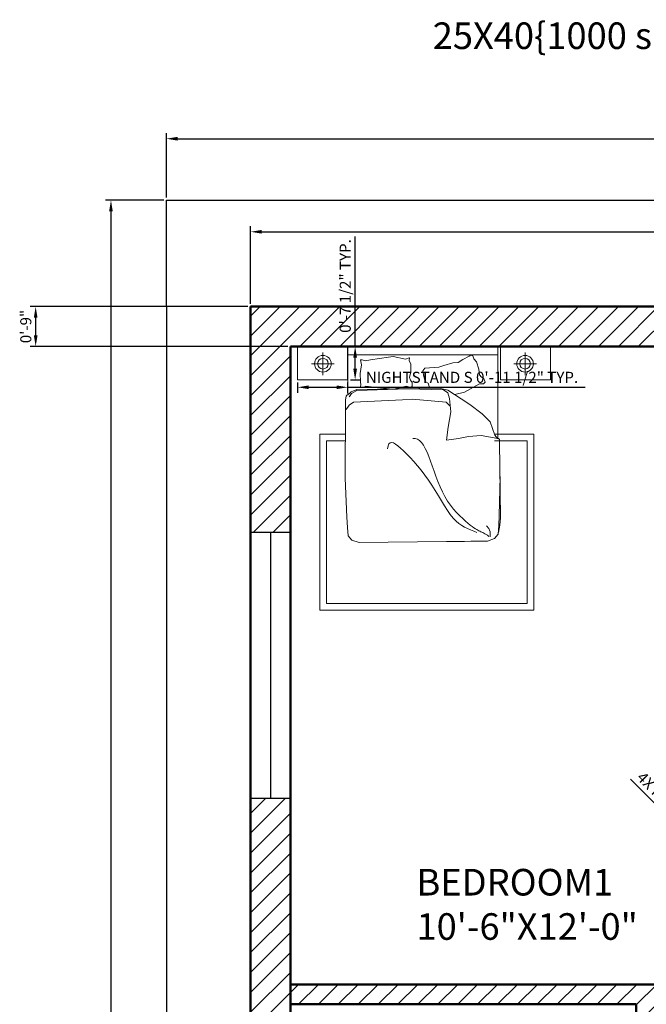
# Model space of a CAD drawing. Units: inches. Extents: x 3542 to 3908, y 2103 to 2666.
# Tile 3 of 4: x 3544 to 3685, y 2444 to 2666. Entities that reach past the tile are written whole.
import ezdxf

# ---------------------------------------------------------------- set-up
doc = ezdxf.new("R2010")
doc.units = ezdxf.units.IN
for name, color, linetype, lineweight in [('A-ANNO-DIMS', 2, 'Continuous', 18), ('A-ANNO-TEXT', 7, 'Continuous', 25), ('A-AREA-IDEN', 7, 'Continuous', 25), ('A-FURN', 8, 'Continuous', 18), ('A-GLAZ', 5, 'Continuous', 25), ('A-WALL', 7, 'Continuous', 50), ('A-WALL-PATT', 252, 'Continuous', 13), ('C-PROP', 7, 'Continuous', 25)]:
    doc.layers.add(name, color=color, linetype=linetype, lineweight=lineweight)
doc.styles.get("Standard").update_dxf_attribs({"font": 'arial.ttf'})
doc.dimstyles.new('ISO-25', dxfattribs={"dimtxt": 2.5, "dimasz": 2.5, "dimexe": 1.25, "dimexo": 0.625, "dimtad": 1, "dimdec": 0, "dimlunit": 3, "dimtxsty": 'Standard', "dimcen": 2.5, "dimadec": 0, "dimazin": 0, "dimtfac": 1, "dimtdec": 0, "dimtmove": 0, "dimatfit": 3, "dimfxl": 1, "dimarcsym": 0})

# ---------------------------------------------------------------- blocks, each defined once
blk = doc.blocks.new('*D8')
at = {"layer": 'A-ANNO-DIMS', "color": 0, "lineweight": -2, "transparency": 16777216}
for p, q in [((3596.14, 2602.1), (3596.14, 2619.62)), ((3598.64, 2618.37), (3862.14, 2618.37)), ((3864.64, 2602.1), (3864.64, 2619.62))]:
    blk.add_line(p, q, dxfattribs=at)
at = {"layer": 'A-ANNO-DIMS', "color": 0, "transparency": 16777216}
for points in [[(3598.64, 2618.79), (3598.64, 2617.96), (3596.14, 2618.37)], [(3862.14, 2618.79), (3862.14, 2617.96), (3864.64, 2618.37)]]:
    blk.add_solid(points, dxfattribs=at)
at = {"layer": 'Defpoints', "color": 0, "transparency": 16777216}
for p in [(3864.64, 2618.37), (3596.14, 2601.48), (3864.64, 2601.48)]:
    blk.add_point(p, dxfattribs=at)
at = {"layer": 'A-ANNO-DIMS', "color": 0, "transparency": 16777216, "insert": (3730.39, 2620.28), "char_height": 2.5, "attachment_point": 5}
blk.add_mtext('22\'-5"', dxfattribs=at)
blk = doc.blocks.new('*D9')
at = {"layer": 'A-ANNO-DIMS', "color": 0, "lineweight": -2, "transparency": 16777216}
for p, q in [((3577.14, 2626.1), (3577.14, 2640.63)), ((3876.64, 2626.1), (3876.64, 2640.63)), ((3579.64, 2639.38), (3874.14, 2639.38))]:
    blk.add_line(p, q, dxfattribs=at)
at = {"layer": 'A-ANNO-DIMS', "color": 0, "transparency": 16777216}
for points in [[(3579.64, 2639.8), (3579.64, 2638.96), (3577.14, 2639.38)], [(3874.14, 2639.8), (3874.14, 2638.96), (3876.64, 2639.38)]]:
    blk.add_solid(points, dxfattribs=at)
at = {"layer": 'Defpoints', "color": 0, "transparency": 16777216}
for p in [(3876.64, 2639.38), (3577.14, 2625.48), (3876.64, 2625.48)]:
    blk.add_point(p, dxfattribs=at)
at = {"layer": 'A-ANNO-DIMS', "color": 0, "transparency": 16777216, "insert": (3726.89, 2641.28), "char_height": 2.5, "attachment_point": 5}
blk.add_mtext("25'", dxfattribs=at)
blk = doc.blocks.new('*D10')
at = {"layer": 'A-ANNO-DIMS', "color": 0, "lineweight": -2, "transparency": 16777216}
for p, q in [((3576.52, 2625.48), (3563.38, 2625.48)), ((3564.63, 2622.98), (3564.63, 2147.48)), ((3576.52, 2144.98), (3563.38, 2144.98))]:
    blk.add_line(p, q, dxfattribs=at)
at = {"layer": 'A-ANNO-DIMS', "color": 0, "transparency": 16777216}
for points in [[(3564.21, 2622.98), (3565.04, 2622.98), (3564.63, 2625.48)], [(3564.21, 2147.48), (3565.04, 2147.48), (3564.63, 2144.98)]]:
    blk.add_solid(points, dxfattribs=at)
at = {"layer": 'Defpoints', "color": 0, "transparency": 16777216}
for p in [(3577.14, 2625.48), (3564.63, 2144.98), (3577.14, 2144.98)]:
    blk.add_point(p, dxfattribs=at)
at = {"layer": 'A-ANNO-DIMS', "color": 0, "transparency": 16777216, "insert": (3562.72, 2385.23), "char_height": 2.5, "attachment_point": 5, "rotation": 90}
blk.add_mtext('40\'-1"', dxfattribs=at)
blk = doc.blocks.new('WIN-60IN')
for p, q in [((0, 60), (0, 0)), ((4.5, 60), (4.5, 0)), ((9, 0), (9, 60))]:
    blk.add_line(p, q)
blk = doc.blocks.new('NIGHTSTAND-SMALL')
for p, q in [((5.7, 6.19), (5.7, 1.07)), ((3.14, 3.63), (8.26, 3.63))]:
    blk.add_line(p, q)
blk.add_lwpolyline([(0, 0), (11.28, 0), (11.28, 7.52), (0, 7.52)], close=True)
for radius in [1.88, 1.2]:
    blk.add_circle((5.7, 3.63), radius)
blk = doc.blocks.new('*D34')
at = {"layer": 'A-ANNO-DIMS', "color": 0, "lineweight": -2, "transparency": 16777216}
for p, q in [((3606.74, 2584.33), (3606.74, 2582.02)), ((3609.24, 2583.27), (3615.52, 2583.27)), ((3618.02, 2584.33), (3618.02, 2582.02)), ((3618.02, 2583.27), (3671.63, 2583.27))]:
    blk.add_line(p, q, dxfattribs=at)
at = {"layer": 'A-ANNO-DIMS', "color": 0, "transparency": 16777216}
for points in [[(3609.24, 2583.68), (3609.24, 2582.85), (3606.74, 2583.27)], [(3615.52, 2583.68), (3615.52, 2582.85), (3618.02, 2583.27)]]:
    blk.add_solid(points, dxfattribs=at)
at = {"layer": 'Defpoints', "color": 0, "transparency": 16777216}
for p in [(3606.74, 2584.96), (3618.02, 2584.96), (3618.02, 2583.27)]:
    blk.add_point(p, dxfattribs=at)
at = {"layer": 'A-ANNO-DIMS', "color": 0, "transparency": 16777216, "insert": (3646.07, 2585.19), "char_height": 2.5, "attachment_point": 5}
blk.add_mtext('NIGHTSTAND S 0\'-11 1/2" TYP.', dxfattribs=at)
blk = doc.blocks.new('*D35')
at = {"layer": 'A-ANNO-DIMS', "color": 0, "lineweight": -2, "transparency": 16777216}
for p, q in [((3619.71, 2592.48), (3619.71, 2617.29)), ((3618.65, 2592.48), (3620.96, 2592.48)), ((3619.71, 2587.46), (3619.71, 2589.98)), ((3618.65, 2584.96), (3620.96, 2584.96))]:
    blk.add_line(p, q, dxfattribs=at)
at = {"layer": 'A-ANNO-DIMS', "color": 0, "transparency": 16777216}
for points in [[(3619.3, 2589.98), (3620.13, 2589.98), (3619.71, 2592.48)], [(3619.3, 2587.46), (3620.13, 2587.46), (3619.71, 2584.96)]]:
    blk.add_solid(points, dxfattribs=at)
at = {"layer": 'Defpoints', "color": 0, "transparency": 16777216}
for p in [(3618.02, 2592.48), (3619.71, 2592.48), (3618.02, 2584.96)]:
    blk.add_point(p, dxfattribs=at)
at = {"layer": 'A-ANNO-DIMS', "color": 0, "transparency": 16777216, "insert": (3617.8, 2606.13), "char_height": 2.5, "attachment_point": 5, "rotation": 90}
blk.add_mtext('0\'-7 1/2" TYP.', dxfattribs=at)
blk = doc.blocks.new('*D50')
at = {"layer": 'A-ANNO-DIMS', "color": 0, "lineweight": -2, "transparency": 16777216}
for p, q in [((3595.52, 2601.48), (3546.39, 2601.48)), ((3547.64, 2598.98), (3547.64, 2594.98)), ((3604.52, 2592.48), (3546.39, 2592.48))]:
    blk.add_line(p, q, dxfattribs=at)
at = {"layer": 'A-ANNO-DIMS', "color": 0, "transparency": 16777216}
for points in [[(3547.23, 2598.98), (3548.06, 2598.98), (3547.64, 2601.48)], [(3547.23, 2594.98), (3548.06, 2594.98), (3547.64, 2592.48)]]:
    blk.add_solid(points, dxfattribs=at)
at = {"layer": 'Defpoints', "color": 0, "transparency": 16777216}
for p in [(3596.14, 2601.48), (3547.64, 2592.48), (3605.14, 2592.48)]:
    blk.add_point(p, dxfattribs=at)
at = {"layer": 'A-ANNO-DIMS', "color": 0, "transparency": 16777216, "insert": (3545.74, 2596.98), "char_height": 2.5, "attachment_point": 5, "rotation": 90}
blk.add_mtext('0\'-9"', dxfattribs=at)
blk = doc.blocks.new('*D65')
at = {"layer": 'A-ANNO-DIMS', "color": 0, "lineweight": -2, "transparency": 16777216}
for p, q in [((3681.84, 2494.78), (3700.92, 2475.7)), ((3728.14, 2448.48), (3702.69, 2473.94))]:
    blk.add_line(p, q, dxfattribs=at)
at = {"layer": 'A-ANNO-DIMS', "color": 0, "transparency": 16777216}
blk.add_solid([(3701.22, 2476), (3700.63, 2475.41), (3702.69, 2473.94)], dxfattribs=at)
at = {"layer": 'Defpoints', "color": 0, "transparency": 16777216}
for p in [(3702.69, 2473.94), (3728.14, 2448.48)]:
    blk.add_point(p, dxfattribs=at)
at = {"layer": 'A-ANNO-DIMS', "color": 0, "transparency": 16777216, "insert": (3688.76, 2490.55), "char_height": 2.5, "attachment_point": 5, "rotation": 314.9996}
blk.add_mtext('4X R3\'-0"', dxfattribs=at)

msp = doc.modelspace()

# ---------------------------------------------------------------- hatches: boundary and pattern name
at = {"layer": 'A-WALL-PATT'}
h = msp.add_hatch(dxfattribs=at)
h.set_pattern_fill('ANSI31', color=256)
h.paths.add_polyline_path([(3864.64, 2601.48), (3596.14, 2601.48), (3596.14, 2550.48), (3605.14, 2550.48), (3605.14, 2592.48), (3855.64, 2592.48), (3855.64, 2550.48), (3864.64, 2550.48)])
h.paths.add_polyline_path([(3735.64, 2592.48), (3731.14, 2592.48), (3731.14, 2448.48), (3728.14, 2448.48), (3728.14, 2443.98), (3738.64, 2443.98), (3738.64, 2448.48), (3735.64, 2448.48)])
h.paths.add_polyline_path([(3855.64, 2448.48), (3774.64, 2448.48), (3774.64, 2443.98), (3855.64, 2443.98)])
h.paths.add_polyline_path([(3605.14, 2490.48), (3596.14, 2490.48), (3596.14, 2426.98), (3605.14, 2426.98)])
h.paths.add_polyline_path([(3605.14, 2402.98), (3596.14, 2402.98), (3596.14, 2350.98), (3605.14, 2350.98)])
h.paths.add_polyline_path([(3692.14, 2448.48), (3605.14, 2448.48), (3605.14, 2443.98), (3683.14, 2443.98), (3683.14, 2440.98), (3687.64, 2440.98), (3687.64, 2443.98), (3692.14, 2443.98)])
h.paths.add_polyline_path([(3687.64, 2404.98), (3683.14, 2404.98), (3683.14, 2385.98), (3605.14, 2385.98), (3605.14, 2381.48), (3687.64, 2381.48)])
h.paths.add_polyline_path([(3864.64, 2490.48), (3855.64, 2490.48), (3855.64, 2397.98), (3864.64, 2397.98)])
h.paths.add_polyline_path([(3864.64, 2337.98), (3855.64, 2337.98), (3855.64, 2269.48), (3864.64, 2269.48)])
h.paths.add_polyline_path([(3864.64, 2233.48), (3855.64, 2233.48), (3855.64, 2215.48), (3831.64, 2215.48), (3831.64, 2206.48), (3864.64, 2206.48)])
h.paths.add_polyline_path([(3771.64, 2215.48), (3740.31, 2215.48), (3740.31, 2206.48), (3771.64, 2206.48)])
h.paths.add_polyline_path([(3747.64, 2287.48), (3750.64, 2287.48), (3750.64, 2291.98), (3743.14, 2291.98), (3743.14, 2215.48), (3747.64, 2215.48)])
h.paths.add_polyline_path([(3706.76, 2215.48), (3695.14, 2215.48), (3695.14, 2291.98), (3690.64, 2291.98), (3690.64, 2206.48), (3690.64, 2158.48), (3665.89, 2158.48), (3665.89, 2153.98), (3690.64, 2153.98), (3699.64, 2153.98), (3699.64, 2206.48), (3706.76, 2206.48)])
h.paths.add_polyline_path([(3605.14, 2314.98), (3596.14, 2314.98), (3596.14, 2153.98), (3629.89, 2153.98), (3629.89, 2158.48), (3605.14, 2158.48)])

# ---------------------------------------------------------------- linework, layer by layer
at = {"layer": 'A-FURN'}
for p, q in [((3618.06, 2581.6), (3618.06, 2592.48)), ((3621.18, 2588.34), (3620.89, 2589.43)), ((3628.29, 2590.2), (3627.27, 2590.09)), ((3631.06, 2589.63), (3628.29, 2590.2)), ((3631.92, 2589.94), (3631.06, 2589.63)), ((3632, 2589.92), (3631.92, 2589.94)), ((3632, 2589.92), (3631.93, 2589.29)), ((3632, 2589.92), (3631.93, 2589.29)), ((3642.93, 2588.86), (3643.98, 2589.56)), ((3642.93, 2588.86), (3643.98, 2589.56)), ((3643.98, 2589.56), (3645.47, 2590.26)), ((3646.48, 2589.67), (3647.08, 2589.02)), ((3631.93, 2589.29), (3632.28, 2588.47)), ((3632.28, 2588.47), (3632.26, 2586.74)), ((3635.44, 2587.62), (3638.62, 2587.81)), ((3638.62, 2587.81), (3639.7, 2588.22)), ((3639.7, 2588.22), (3641.73, 2588.76)), ((3641.73, 2588.76), (3642.93, 2588.86)), ((3647.08, 2589.02), (3647.65, 2587.39)), ((3647.65, 2587.39), (3647.8, 2586.08)), ((3632.26, 2586.74), (3631.95, 2585.46)), ((3631.95, 2585.46), (3632.17, 2584.84)), ((3647.8, 2586.08), (3648.21, 2585.57)), ((3648.21, 2585.57), (3648.73, 2585.24)), ((3648.73, 2585.24), (3649.08, 2584.41)), ((3631.2, 2583.55), (3628.46, 2582.85)), ((3632.07, 2583.28), (3631.2, 2583.55)), ((3632.6, 2583.45), (3632.07, 2583.28)), ((3632.17, 2584.84), (3632.54, 2584.36)), ((3632.54, 2584.36), (3632.6, 2583.45)), ((3647.73, 2584.03), (3644.4, 2582.16)), ((3648.64, 2584.07), (3647.73, 2584.03)), ((3649.08, 2584.41), (3648.64, 2584.07)), ((3617.59, 2580.85), (3617.54, 2580.33)), ((3617.56, 2579.1), (3617.49, 2562.72)), ((3617.54, 2580.33), (3617.56, 2579.1)), ((3651.85, 2571.71), (3651.92, 2571.74)), ((3652.36, 2565.41), (3652.3, 2570.73)), ((3652.48, 2553.78), (3652.36, 2565.41)), ((3652.4, 2563.13), (3652.17, 2554.34)), ((3617.49, 2562.72), (3617.84, 2553.94)), ((3617.84, 2553.94), (3617.96, 2551.64)), ((3652.17, 2554.34), (3652.12, 2552.04)), ((3649.88, 2551.39), (3649.33, 2551.97)), ((3652.12, 2552.04), (3651.97, 2550.14)), ((3652.06, 2550.48), (3652.38, 2552.16)), ((3652.38, 2552.16), (3652.48, 2553.78)), ((3617.96, 2551.64), (3618.17, 2549.74)), ((3618.17, 2549.74), (3619, 2548.74)), ((3650.14, 2550.62), (3649.88, 2551.39)), ((3650.19, 2549.5), (3650.14, 2550.62)), ((3651.97, 2550.14), (3651.17, 2549.11)), ((3619, 2548.74), (3620.6, 2548.2)), ((3640.35, 2548.42), (3620.6, 2548.2)), ((3640.35, 2548.42), (3644.39, 2548.42)), ((3644.39, 2548.42), (3645.81, 2548.52)), ((3645.81, 2548.52), (3649.58, 2548.52)), ((3651.17, 2549.11), (3649.58, 2548.52))]:
    msp.add_line(p, q, dxfattribs=at)
for points in [[(3618.06, 2592.48), (3651.91, 2592.48), (3651.91, 2571.77)], [(3651.91, 2590.6), (3618.06, 2590.6)], [(3627.27, 2590.09), (3623.17, 2589.47), (3621.99, 2589.27), (3621.28, 2589.5), (3620.89, 2589.43)], [(3646.48, 2589.67), (3646.27, 2590.37), (3645.82, 2590.51), (3645.47, 2590.26)], [(3627.43, 2582.92), (3623.31, 2583.35), (3622.11, 2583.5), (3621.42, 2583.24), (3620.84, 2583.31), (3621, 2583.77), (3620.91, 2584.55), (3620.88, 2586.36), (3621.14, 2588.34)], [(3635.44, 2587.62), (3635.01, 2587), (3635.22, 2585.69), (3635.53, 2584.54), (3636.16, 2584.17), (3636.52, 2583.23), (3636.53, 2583.06)], [(3651.91, 2571.7), (3648.12, 2572.36), (3645.32, 2572.15), (3643.03, 2571.69), (3640.32, 2571.31), (3640.68, 2574.27), (3641.29, 2577.71), (3641.03, 2580.76), (3640.63, 2581.99), (3639.64, 2582.69), (3631.62, 2582.91), (3620.08, 2582.57), (3618.9, 2581.87), (3618.41, 2581.18), (3618.34, 2581.11)], [(3618.35, 2581.8), (3618.81, 2582.21), (3620.08, 2582.74), (3638.78, 2583.1), (3640.66, 2582.62), (3643.66, 2580.63), (3645.55, 2579.38), (3648.38, 2577.3), (3650.2, 2575.45), (3651.26, 2572.49), (3651.79, 2571.72)], [(3617.6, 2580.89), (3617.71, 2581.24), (3617.87, 2581.51), (3618.06, 2581.6), (3618.28, 2581.79), (3618.32, 2581.81)], [(3641.07, 2579.08), (3640.22, 2579.94), (3632.58, 2580.59), (3630.36, 2580.46), (3619.31, 2579.9), (3618.38, 2579.2), (3617.67, 2578.26)], [(3644.4, 2582.16), (3642.18, 2581.61)], [(3651.18, 2572.71), (3660.03, 2572.71), (3660.03, 2532.97), (3611.78, 2532.97), (3611.78, 2572.71), (3617.53, 2572.71)], [(3649.85, 2549.62), (3649.54, 2549.86), (3649.25, 2550.06), (3648.99, 2550.22), (3648.75, 2550.35), (3648.53, 2550.47), (3648.31, 2550.57), (3648.09, 2550.67), (3647.87, 2550.76), (3647.64, 2550.87), (3647.4, 2550.99), (3647.13, 2551.14), (3646.83, 2551.32), (3646.49, 2551.54), (3646.11, 2551.82), (3645.67, 2552.16), (3645.16, 2552.57), (3644.59, 2553.05), (3643.97, 2553.62), (3643.3, 2554.26), (3642.61, 2554.98), (3641.92, 2555.77), (3641.24, 2556.64), (3640.58, 2557.58), (3639.96, 2558.6), (3639.39, 2559.68), (3638.87, 2560.82), (3638.39, 2561.99), (3637.95, 2563.18), (3637.53, 2564.36), (3637.12, 2565.51), (3636.73, 2566.62), (3636.34, 2567.66), (3635.94, 2568.61), (3635.53, 2569.47), (3635.11, 2570.21), (3634.67, 2570.82), (3634.22, 2571.29), (3633.75, 2571.59), (3633.26, 2571.73), (3632.75, 2571.67)], [(3652.3, 2570.78), (3652.25, 2571.51), (3652.04, 2571.73), (3651.91, 2571.77)], [(3651.18, 2571.2), (3658.53, 2571.2), (3658.53, 2534.47), (3613.28, 2534.47), (3613.28, 2571.2), (3617.53, 2571.2)], [(3647.18, 2550.51), (3646.46, 2550.82), (3645.76, 2551.11), (3645.08, 2551.4), (3644.42, 2551.72), (3643.76, 2552.08), (3643.11, 2552.52), (3642.47, 2553.06), (3641.83, 2553.72), (3641.18, 2554.53), (3640.53, 2555.46), (3639.86, 2556.49), (3639.19, 2557.6), (3638.49, 2558.76), (3637.77, 2559.95), (3637.02, 2561.15), (3636.25, 2562.32), (3635.44, 2563.45), (3634.61, 2564.53), (3633.77, 2565.55), (3632.94, 2566.51), (3632.13, 2567.39), (3631.35, 2568.19), (3630.61, 2568.9), (3629.94, 2569.52), (3629.33, 2570.04), (3628.79, 2570.43), (3628.33, 2570.69), (3627.93, 2570.79), (3627.6, 2570.73), (3627.33, 2570.48), (3627.13, 2570.03), (3627, 2569.35)]]:
    msp.add_lwpolyline(points, dxfattribs=at)
at = {"layer": 'A-GLAZ'}
for p, q in [((3605.14, 2550.48), (3596.14, 2550.48)), ((3596.14, 2490.48), (3605.14, 2490.48))]:
    msp.add_line(p, q, dxfattribs=at)
at = {"layer": 'A-WALL'}
for p, q in [((3596.14, 2601.48), (3596.14, 2153.98)), ((3596.14, 2601.48), (3864.64, 2601.48)), ((3596.14, 2601.48), (3864.64, 2601.48)), ((3605.14, 2592.48), (3855.64, 2592.48)), ((3605.14, 2592.48), (3605.14, 2158.48)), ((3605.14, 2448.48), (3692.14, 2448.48)), ((3605.14, 2443.98), (3683.14, 2443.98)), ((3683.14, 2443.98), (3683.14, 2440.98))]:
    msp.add_line(p, q, dxfattribs=at)
at = {"layer": 'C-PROP'}
for p, q in [((3577.14, 2601.48), (3577.14, 2625.48)), ((3577.14, 2625.48), (3596.14, 2625.48)), ((3596.14, 2625.48), (3864.64, 2625.48)), ((3577.14, 2601.48), (3577.14, 2144.98))]:
    msp.add_line(p, q, dxfattribs=at)

# ---------------------------------------------------------------- block references
at = {"layer": 'A-FURN'}
msp.add_blockref('NIGHTSTAND-SMALL', (3606.74, 2584.96), dxfattribs=at)
at = {"layer": 'A-FURN', "extrusion": (0, 0, -1), "zscale": -1}
msp.add_blockref('NIGHTSTAND-SMALL', (-3663.75, 2584.96), dxfattribs=at)
at = {"layer": 'A-GLAZ'}
msp.add_blockref('WIN-60IN', (3596.14, 2490.48), dxfattribs=at)

# ---------------------------------------------------------------- texts
at = {"layer": 'A-ANNO-TEXT', "insert": (3637.21, 2665.63), "char_height": 6, "width": 219.7452, "attachment_point": 1}
msp.add_mtext('25X40\\{1000 sq ft\\}HOUSE PLAN-WEST FACE-FP1325', dxfattribs=at)
at = {"layer": 'A-AREA-IDEN', "insert": (3633.55, 2474.54), "char_height": 6, "attachment_point": 1}
msp.add_mtext('BEDROOM1\\P10\'-6"X12\'-0"', dxfattribs=at)

# ---------------------------------------------------------------- dimensions: what is measured, and where the dimension line sits
at = {"layer": 'A-ANNO-DIMS'}
for base, p1, p2, picture, middle in [((3876.64448065, 2639.37837652), (3577.14448065, 2625.47915136), (3876.64448065, 2625.47915136), '*D9', (3726.89448065, 2641.27980899)), ((3864.64448065, 2618.37377621), (3596.14448065, 2601.47915136), (3864.64448065, 2601.47915136), '*D8', (3730.39448065, 2620.27520868))]:
    dim = msp.add_linear_dim(base=base, p1=p1, p2=p2, dimstyle='ISO-25', override={"dimclrd": 0, "dimclre": 0, "dimclrt": 0}, dxfattribs=at)
    dim.commit()
    dim.dimension.update_dxf_attribs({"geometry": picture, "text_midpoint": middle})
for base, p1, p2, override, picture, middle in [((3564.62592245, 2144.97915136), (3577.14448065, 2625.47915136), (3577.14448065, 2144.97915136), {"dimclrd": 0, "dimclre": 0, "dimclrt": 0}, '*D10', (3562.72448998, 2385.22915136)), ((3547.64, 2592.48), (3596.14, 2601.48), (3605.14, 2592.48), {"dimdec": 1, "dimlfac": 1, "dimrnd": 0, "dimzin": 1, "dimdsep": 46, "dimlunit": 4, "dimfrac": 2}, '*D50', (3545.74, 2596.98))]:
    dim = msp.add_linear_dim(base=base, p1=p1, p2=p2, angle=90, dimstyle='ISO-25', override=override, dxfattribs=at)
    dim.commit()
    dim.dimension.update_dxf_attribs({"geometry": picture, "text_midpoint": middle})
dim = msp.add_linear_dim(base=(3619.71, 2592.48), p1=(3618.02, 2584.96), p2=(3618.02, 2592.48), angle=90, text='<> TYP.', dimstyle='ISO-25', override={"dimdec": 1, "dimlfac": 1, "dimrnd": 0, "dimzin": 1, "dimdsep": 46, "dimlunit": 4, "dimfrac": 2}, dxfattribs=at)
dim.commit()
dim.dimension.update_dxf_attribs({"geometry": '*D35', "text_midpoint": (3617.8, 2606.13)})
dim = msp.add_linear_dim(base=(3618.02, 2583.27), p1=(3606.74, 2584.96), p2=(3618.02, 2584.96), text='NIGHTSTAND S <> TYP.', dimstyle='ISO-25', override={"dimdec": 1, "dimlfac": 1, "dimrnd": 0, "dimzin": 1, "dimdsep": 46, "dimlunit": 4, "dimfrac": 2}, dxfattribs=at)
dim.commit()
dim.dimension.update_dxf_attribs({"geometry": '*D34', "text_midpoint": (3646.07, 2585.19)})
dim = msp.add_radius_dim(center=(3728.14, 2448.48), mpoint=(3702.69, 2473.94), text='4X <>', dimstyle='ISO-25', override={"dimdec": 1, "dimlfac": 1, "dimrnd": 0, "dimzin": 1, "dimdsep": 46, "dimlunit": 4, "dimfrac": 2}, dxfattribs=at)
dim.commit()
dim.dimension.update_dxf_attribs({"geometry": '*D65', "text_midpoint": (3687.42, 2489.21), "dimtype": 164})

doc.saveas('drawing.dxf')
